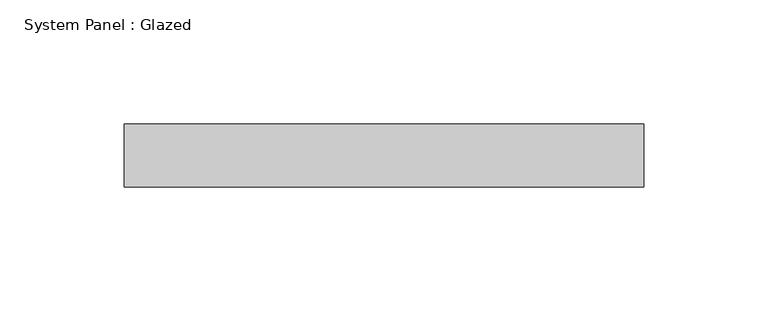
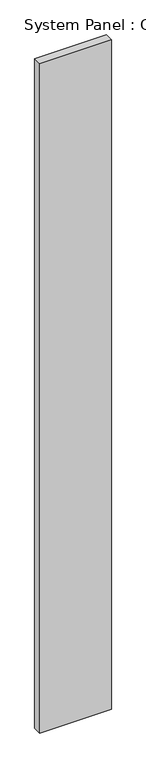
"""IFC4 building model written with IfcOpenShell, lengths in millimetres: plate geometry, System Panel : Glazed."""

from ifc_helpers import new_model, si_unit, origin, origin_with_axes, place, context, project, spatial, polyline, outline, extrude, source, transform, mapped, element, save


def system_panel_glazed_b82c55cd(model_context):
    return source(origin(), model_context, "Body", "SweptSolid", [
        extrude(outline(polyline([(104.775, 19.05), (-104.775, 19.05), (-104.775, 44.45), (104.775, 44.45), (104.775, 19.05)])), origin_with_axes(), (0.0, 0.0, 1.0), 2070.1),
    ])


if __name__ == "__main__":
    model = new_model("IFC4")
    model_context = context("Model", 3, world=origin())
    ifc_project = project(units=[si_unit("LENGTHUNIT", "METRE", prefix="MILLI")], contexts=[model_context])
    site = spatial("IfcSite", under=ifc_project)
    building = spatial("IfcBuilding", under=site)
    placement = place(None, origin())
    system_panel_glazed_shape = system_panel_glazed_b82c55cd(model_context)
    element("IfcPlate", 1, ObjectType="System Panel : Glazed", at=placement, inside=building, context=model_context, shape_type="MappedRepresentation", body=[
        mapped(system_panel_glazed_shape, transform((0.0, 0.0, 0.0), x_axis=(1.0, 0.0, 0.0), y_axis=(0.0, 1.0, 0.0), z_axis=(0.0, 0.0, 1.0))),
    ])
    save(model, "model.ifc")

# Revit data of these elements
# Type "System Panel : Glazed"
#   Construction Type Id = "GSP4R"
#   Analytic Construction = "1/8 in Pilkington single glazing"
#   Visual Light Transmittance = 0.9
#   Solar Heat Gain Coefficient = 0.86
#   Heat Transfer Coefficient (U) = 1.18115 BTU/(h·ft²·°F)
#   Define Thermal Properties by = 1
# Element 1 (IfcPlate, "System Panel : Glazed")
#   Materials on its faces: "Glass"
# Materials
#   "Glass": class "Glass", colour RGB 0 128 192, transparency 0.75, Description = "Soda Lime Glass", Cost = 0
